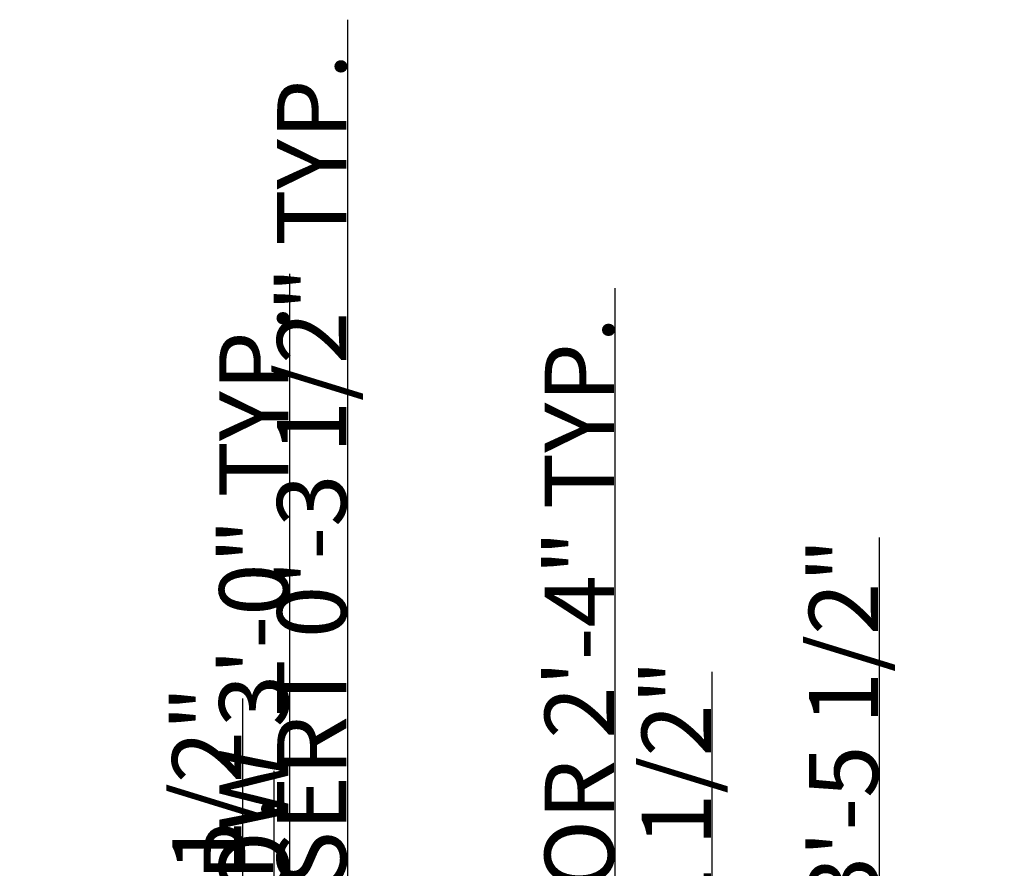
# Model space of a CAD drawing. Units: inches. Extents: x 2236 to 2927, y 1577 to 2452.
# Tile 9 of 9: x 2308 to 2649, y 2157 to 2452. Entities that reach past the tile are written whole.
import ezdxf

# ---------------------------------------------------------------- set-up
doc = ezdxf.new("R2010")
doc.units = ezdxf.units.IN
doc.layers.add('A-ANNO-DIMS', color=2, linetype='Continuous', lineweight=18)
doc.styles.get("Standard").update_dxf_attribs({"font": 'arial.ttf'})
doc.dimstyles.get("Standard").update_dxf_attribs({"dimtxt": 24, "dimasz": 12, "dimexe": 0.18, "dimexo": 0.0625, "dimgap": 0.09, "dimtad": 1, "dimdec": 1, "dimzin": 0, "dimdsep": 46, "dimlunit": 4, "dimtxsty": 'Standard', "dimcen": 0.09, "dimadec": 0, "dimazin": 0, "dimtfac": 1, "dimtdec": 1, "dimtofl": 0, "dimtmove": 0, "dimatfit": 3, "dimfxl": 1, "dimtolj": 1, "dimtzin": 0, "dimarcsym": 0})

# ---------------------------------------------------------------- blocks, each defined once
blk = doc.blocks.new('*D16')
at = {"layer": 'A-ANNO-DIMS', "color": 0, "lineweight": -2, "transparency": 16777216}
for p, q in [((2421.54, 1988.01), (2421.54, 2451.93)), ((2421.05, 1976.01), (2421.72, 1976.01)), ((2421.05, 1972.34), (2421.72, 1972.34)), ((2421.54, 1960.34), (2421.54, 1948.34))]:
    blk.add_line(p, q, dxfattribs=at)
at = {"layer": 'A-ANNO-DIMS', "color": 0, "transparency": 16777216}
for points in [[(2419.54, 1988.01), (2423.54, 1988.01), (2421.54, 1976.01)], [(2419.54, 1960.34), (2423.54, 1960.34), (2421.54, 1972.34)]]:
    blk.add_solid(points, dxfattribs=at)
at = {"layer": 'Defpoints', "color": 0, "transparency": 16777216}
for p in [(2420.99, 1976.01), (2421.54, 1976.01), (2420.99, 1972.34)]:
    blk.add_point(p, dxfattribs=at)
at = {"layer": 'A-ANNO-DIMS', "color": 0, "transparency": 16777216, "insert": (2409.03, 2225.97), "char_height": 24, "attachment_point": 5, "rotation": 90}
blk.add_mtext('\\A1;SHELF INSERT 0\'-3 1/2" TYP.', dxfattribs=at)
blk = doc.blocks.new('*D18')
at = {"layer": 'A-ANNO-DIMS', "color": 0, "lineweight": -2, "transparency": 16777216}
for p, q in [((2396.05, 1834.44), (2396.05, 2191.28)), ((2406.79, 1834.44), (2395.87, 1834.44)), ((2396.05, 1774.44), (2396.05, 1822.44)), ((2406.79, 1762.44), (2395.87, 1762.44))]:
    blk.add_line(p, q, dxfattribs=at)
at = {"layer": 'A-ANNO-DIMS', "color": 0, "transparency": 16777216}
for points in [[(2394.05, 1822.44), (2398.05, 1822.44), (2396.05, 1834.44)], [(2394.05, 1774.44), (2398.05, 1774.44), (2396.05, 1762.44)]]:
    blk.add_solid(points, dxfattribs=at)
at = {"layer": 'Defpoints', "color": 0, "transparency": 16777216}
for p in [(2396.05, 1834.44), (2406.85, 1834.44), (2406.85, 1762.44)]:
    blk.add_point(p, dxfattribs=at)
at = {"layer": 'A-ANNO-DIMS', "color": 0, "transparency": 16777216, "insert": (2383.54, 2018.86), "char_height": 24, "attachment_point": 5, "rotation": 90}
blk.add_mtext('\\A1;WINDOW W 6\'-0" TYP.', dxfattribs=at)
blk = doc.blocks.new('*D20')
at = {"layer": 'A-ANNO-DIMS', "color": 0, "lineweight": -2, "transparency": 16777216}
for p, q in [((2401.45, 1929.71), (2401.45, 2363.75)), ((2406.79, 1929.71), (2401.27, 1929.71)), ((2401.45, 1905.71), (2401.45, 1917.71)), ((2406.79, 1893.71), (2401.27, 1893.71))]:
    blk.add_line(p, q, dxfattribs=at)
at = {"layer": 'A-ANNO-DIMS', "color": 0, "transparency": 16777216}
for points in [[(2399.45, 1917.71), (2403.45, 1917.71), (2401.45, 1929.71)], [(2399.45, 1905.71), (2403.45, 1905.71), (2401.45, 1893.71)]]:
    blk.add_solid(points, dxfattribs=at)
at = {"layer": 'Defpoints', "color": 0, "transparency": 16777216}
for p in [(2401.45, 1929.71), (2406.85, 1929.71), (2406.85, 1893.71)]:
    blk.add_point(p, dxfattribs=at)
at = {"layer": 'A-ANNO-DIMS', "color": 0, "transparency": 16777216, "insert": (2388.93, 2152.73), "char_height": 24, "attachment_point": 5, "rotation": 90}
blk.add_mtext('\\A1;SMALL WINDOW 3\'-0" TYP.', dxfattribs=at)
blk = doc.blocks.new('*D22')
at = {"layer": 'A-ANNO-DIMS', "color": 0, "lineweight": -2, "transparency": 16777216}
for p, q in [((2514.42, 1977.96), (2514.42, 2358.7)), ((2518.53, 1977.96), (2514.24, 1977.96)), ((2514.42, 1962.08), (2514.42, 1965.96)), ((2518.53, 1950.08), (2514.24, 1950.08))]:
    blk.add_line(p, q, dxfattribs=at)
at = {"layer": 'A-ANNO-DIMS', "color": 0, "transparency": 16777216}
for points in [[(2512.42, 1965.96), (2516.42, 1965.96), (2514.42, 1977.96)], [(2512.42, 1962.08), (2516.42, 1962.08), (2514.42, 1950.08)]]:
    blk.add_solid(points, dxfattribs=at)
at = {"layer": 'Defpoints', "color": 0, "transparency": 16777216}
for p in [(2514.42, 1977.96), (2518.6, 1977.96), (2518.6, 1950.08)]:
    blk.add_point(p, dxfattribs=at)
at = {"layer": 'A-ANNO-DIMS', "color": 0, "transparency": 16777216, "insert": (2501.91, 2174.33), "char_height": 24, "attachment_point": 5, "rotation": 90}
blk.add_mtext('\\A1;ROOM DOOR 2\'-4" TYP.', dxfattribs=at)
blk = doc.blocks.new('*D29')
at = {"layer": 'A-ANNO-DIMS', "color": 0, "lineweight": -2, "transparency": 16777216}
for p, q in [((2548.08, 2075.08), (2548.08, 2225.62)), ((2532.86, 2075.08), (2548.26, 2075.08)), ((2548.08, 2015.35), (2548.08, 2063.08)), ((2532.86, 2003.35), (2548.26, 2003.35))]:
    blk.add_line(p, q, dxfattribs=at)
at = {"layer": 'A-ANNO-DIMS', "color": 0, "transparency": 16777216}
for points in [[(2546.08, 2063.08), (2550.08, 2063.08), (2548.08, 2075.08)], [(2546.08, 2015.35), (2550.08, 2015.35), (2548.08, 2003.35)]]:
    blk.add_solid(points, dxfattribs=at)
at = {"layer": 'Defpoints', "color": 0, "transparency": 16777216}
for p in [(2532.8, 2075.08), (2548.08, 2075.08), (2532.8, 2003.35)]:
    blk.add_point(p, dxfattribs=at)
at = {"layer": 'A-ANNO-DIMS', "color": 0, "transparency": 16777216, "insert": (2535.58, 2156.35), "char_height": 24, "attachment_point": 5, "rotation": 90}
blk.add_mtext('\\A1;5\'-11 1/2"', dxfattribs=at)
blk = doc.blocks.new('*D30')
at = {"layer": 'A-ANNO-DIMS', "color": 0, "lineweight": -2, "transparency": 16777216}
for p, q in [((2606.12, 2074.13), (2606.12, 2272.19)), ((2599.94, 2074.13), (2606.3, 2074.13)), ((2606.12, 2044.51), (2606.12, 2062.13)), ((2599.94, 2032.51), (2606.3, 2032.51))]:
    blk.add_line(p, q, dxfattribs=at)
at = {"layer": 'A-ANNO-DIMS', "color": 0, "transparency": 16777216}
for points in [[(2604.12, 2062.13), (2608.12, 2062.13), (2606.12, 2074.13)], [(2604.12, 2044.51), (2608.12, 2044.51), (2606.12, 2032.51)]]:
    blk.add_solid(points, dxfattribs=at)
at = {"layer": 'Defpoints', "color": 0, "transparency": 16777216}
for p in [(2599.88, 2074.13), (2606.12, 2074.13), (2599.88, 2032.51)]:
    blk.add_point(p, dxfattribs=at)
at = {"layer": 'A-ANNO-DIMS', "color": 0, "transparency": 16777216, "insert": (2593.61, 2179.16), "char_height": 24, "attachment_point": 5, "rotation": 90}
blk.add_mtext('\\A1;WC 3\'-5 1/2"', dxfattribs=at)
blk = doc.blocks.new('*D42')
at = {"layer": 'A-ANNO-DIMS', "color": 0, "lineweight": -2, "transparency": 16777216}
for p, q in [((2385.1, 2084.08), (2385.1, 2216.39)), ((2406.79, 2084.08), (2384.92, 2084.08)), ((2385.1, 2064.78), (2385.1, 2072.08)), ((2406.79, 2052.78), (2384.92, 2052.78))]:
    blk.add_line(p, q, dxfattribs=at)
at = {"layer": 'A-ANNO-DIMS', "color": 0, "transparency": 16777216}
for points in [[(2383.1, 2072.08), (2387.1, 2072.08), (2385.1, 2084.08)], [(2383.1, 2064.78), (2387.1, 2064.78), (2385.1, 2052.78)]]:
    blk.add_solid(points, dxfattribs=at)
at = {"layer": 'Defpoints', "color": 0, "transparency": 16777216}
for p in [(2385.1, 2084.08), (2406.85, 2084.08), (2406.85, 2052.78)]:
    blk.add_point(p, dxfattribs=at)
at = {"layer": 'A-ANNO-DIMS', "color": 0, "transparency": 16777216, "insert": (2372.6, 2156.23), "char_height": 24, "attachment_point": 5, "rotation": 90}
blk.add_mtext('\\A1;2\'-7 1/2"', dxfattribs=at)

msp = doc.modelspace()

# ---------------------------------------------------------------- dimensions: what is measured, and where the dimension line sits
at = {"layer": 'A-ANNO-DIMS'}
for base, p1, p2, text, picture, middle in [((2421.54, 1976.01), (2420.99, 1972.34), (2420.99, 1976.01), 'SHELF INSERT <> TYP.', '*D16', (2409.03, 2225.97)), ((2401.45, 1929.71), (2406.85, 1893.71), (2406.85, 1929.71), 'SMALL WINDOW <> TYP.', '*D20', (2388.93, 2152.73)), ((2514.42, 1977.96), (2518.6, 1950.08), (2518.6, 1977.96), 'ROOM DOOR <> TYP.', '*D22', (2501.91, 2174.33)), ((2606.12, 2074.13), (2599.88, 2032.51), (2599.88, 2074.13), 'WC <>', '*D30', (2593.61, 2179.16)), ((2396.05, 1834.44), (2406.85, 1762.44), (2406.85, 1834.44), 'WINDOW W <> TYP.', '*D18', (2383.54, 2018.86))]:
    dim = msp.add_linear_dim(base=base, p1=p1, p2=p2, angle=90, text=text, dimstyle='Standard', override={"dimdec": 1, "dimlfac": 1, "dimrnd": 0, "dimzin": 1, "dimdsep": 46, "dimlunit": 4, "dimfrac": 2}, dxfattribs=at)
    dim.commit()
    dim.dimension.update_dxf_attribs({"geometry": picture, "text_midpoint": middle})
for base, p1, p2, picture, middle in [((2548.08, 2075.08), (2532.8, 2003.35), (2532.8, 2075.08), '*D29', (2535.58, 2156.35)), ((2385.1, 2084.08), (2406.85, 2052.78), (2406.85, 2084.08), '*D42', (2372.6, 2156.23))]:
    dim = msp.add_linear_dim(base=base, p1=p1, p2=p2, angle=90, dimstyle='Standard', override={"dimdec": 1, "dimlfac": 1, "dimrnd": 0, "dimzin": 1, "dimdsep": 46, "dimlunit": 4, "dimfrac": 2}, dxfattribs=at)
    dim.commit()
    dim.dimension.update_dxf_attribs({"geometry": picture, "text_midpoint": middle})

doc.saveas('drawing.dxf')
